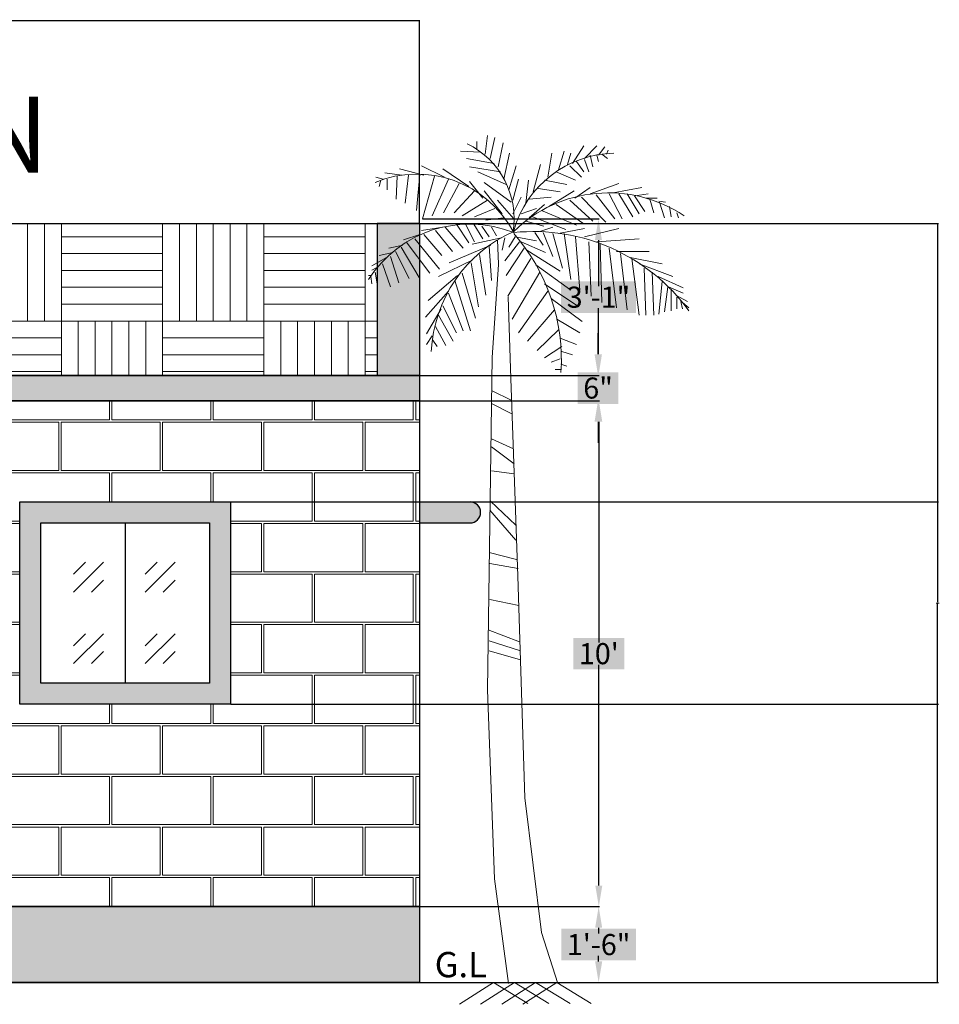
# Model space of a CAD drawing. Units: inches. Extents: x -301 to 715, y -607 to 364.
# Tile 139 of 141: x 497 to 715, y -513 to -279. Entities that reach past the tile are written whole.
import ezdxf

# ---------------------------------------------------------------- set-up
doc = ezdxf.new("R2010")
doc.units = ezdxf.units.IN
doc.header["$MEASUREMENT"] = 0
for name, color, linetype, lineweight in [('A-ANNO-DIMS', 2, 'Continuous', 18), ('A-ANNO-SYMB', 4, 'Continuous', 18), ('A-ANNO-TITL', 1, 'Continuous', 35), ('A-ELEV', 220, 'Continuous', 30), ('A-ELEV-PATT', 4, 'Continuous', 13), ('A-GLAZ', 2, 'Continuous', 25), ('A-GRND', 7, 'Continuous', 25), ('L-PLNT', 94, 'Continuous', 13)]:
    doc.layers.add(name, color=color, linetype=linetype, lineweight=lineweight)
doc.styles.get("Standard").update_dxf_attribs({"font": 'arial.ttf'})
doc.dimstyles.get("Standard").update_dxf_attribs({"dimtxt": 0.18, "dimasz": 0.18, "dimexe": 0.18, "dimexo": 0.0625, "dimgap": 0.09, "dimtad": 0, "dimtih": 1, "dimtoh": 1, "dimdec": 1, "dimzin": 0, "dimdsep": 46, "dimlunit": 4, "dimtxsty": 'Standard', "dimcen": 0.09, "dimclrd": 3, "dimclre": 4, "dimclrt": 6, "dimadec": 0, "dimazin": 0, "dimtfac": 1, "dimtdec": 1, "dimtofl": 0, "dimtmove": 0, "dimatfit": 3, "dimfxl": 1, "dimtfill": 2, "dimtfillclr": 51, "dimtolj": 1, "dimtzin": 0, "dimarcsym": 0})

# ---------------------------------------------------------------- blocks, each defined once
blk = doc.blocks.new('*U34')
for p, q in [((-5.567, 196.707), (-4.987, 201.167)), ((-7.5, 199.68), (-7.5, 197.946)), ((-4.407, 195.716), (-3.247, 200.672)), ((-2.474, 193.733), (-1.315, 199.433)), ((15.116, 194.477), (17.822, 198.689)), ((18.015, 195.716), (20.914, 198.689)), ((-6.727, 197.202), (-11.366, 197.45)), ((-1.121, 190.759), (0.232, 196.955)), ((9.317, 191.255), (10.283, 196.955)), ((11.829, 192.99), (13.182, 197.45)), ((13.956, 194.229), (14.729, 196.955)), ((19.368, 196.459), (19.948, 193.733)), ((20.914, 196.459), (21.301, 194.972)), ((21.301, 196.459), (22.847, 198.441)), ((22.074, 196.707), (23.427, 195.716)), ((23.234, 196.707), (23.62, 197.698)), ((-15.232, 191.255), (-20.644, 193.981)), ((-3.441, 194.477), (-10.013, 195.716)), ((0.038, 188.281), (1.778, 193.981)), ((5.837, 187.786), (7.577, 194.229)), ((14.536, 193.981), (17.242, 191.255)), ((16.082, 194.972), (17.822, 192.494)), ((18.015, 195.468), (18.981, 192.494)), ((-25.283, 191.751), (-29.342, 192.246)), ((-26.443, 191.503), (-26.636, 186.051)), ((-20.064, 191.751), (-25.863, 193.238)), ((-23.737, 191.751), (-24.51, 185.06)), ((-21.031, 191.998), (-21.804, 183.325)), ((-17.551, 191.503), (-20.451, 181.343)), ((-9.433, 189.025), (-15.618, 193.238)), ((-1.894, 192.494), (-9.24, 193.733)), ((-0.541, 189.52), (-7.307, 192.494)), ((11.25, 192.494), (15.889, 190.512)), ((-29.729, 190.759), (-31.469, 191.255)), ((-30.309, 190.512), (-30.695, 189.025)), ((-28.763, 190.759), (-28.763, 188.281)), ((-14.265, 190.759), (-18.131, 182.086)), ((-11.753, 189.768), (-15.425, 182.83)), ((-6.147, 186.299), (-9.24, 190.264)), ((-5.76, 190.016), (0.618, 185.308)), ((1.005, 185.803), (2.358, 190.759)), ((4.098, 185.06), (4.678, 190.512)), ((8.544, 190.512), (13.763, 189.52)), ((19.368, 187.29), (26.133, 189.768)), ((-8.08, 188.034), (-12.912, 182.83)), ((-5.76, 188.034), (-1.508, 182.582)), ((6.997, 188.529), (12.216, 187.786)), ((9.51, 184.317), (15.502, 188.034)), ((15.695, 186.299), (19.368, 188.777)), ((20.721, 187.042), (25.167, 181.343)), ((23.814, 187.29), (26.907, 181.343)), ((24.78, 187.538), (31.546, 188.777)), ((26.133, 187.29), (29.419, 181.838)), ((28.066, 187.29), (30.966, 182.582)), ((29.999, 186.795), (33.092, 187.29)), ((-4.987, 185.803), (-10.979, 182.086)), ((-2.668, 185.803), (1.198, 181.343)), ((1.005, 182.582), (2.938, 186.547)), ((4.871, 186.051), (10.09, 186.547)), ((4.871, 181.591), (8.544, 184.812)), ((11.25, 184.812), (17.628, 180.352)), ((14.536, 185.803), (19.948, 180.847)), ((17.242, 186.547), (23.041, 180.599)), ((29.806, 186.795), (32.319, 183.078)), ((32.512, 186.299), (35.218, 186.299)), ((33.479, 186.051), (34.445, 182.83)), ((35.605, 185.556), (37.151, 185.308)), ((35.798, 185.308), (36.958, 181.591)), ((-3.247, 183.821), (-8.08, 181.838)), ((2.938, 182.582), (6.61, 183.821)), ((7.77, 183.325), (16.082, 179.856)), ((38.118, 184.317), (38.504, 181.838)), ((39.857, 182.83), (40.244, 181.591)), ((-12.332, 180.104), (-9.433, 175.643)), ((-10.206, 180.104), (-8.08, 175.891)), ((-8.273, 180.104), (-6.147, 176.635)), ((-1.315, 181.591), (-5.374, 181.095)), ((-0.348, 180.352), (-1.894, 180.104)), ((4.098, 180.847), (8.35, 179.608)), ((5.644, 181.838), (13.569, 178.865)), ((-21.031, 177.626), (-24.897, 176.387)), ((-15.618, 179.36), (-20.644, 178.617)), ((-20.064, 177.626), (-15.812, 172.67)), ((-17.358, 178.617), (-13.299, 173.661)), ((-15.038, 179.36), (-10.786, 174.404)), ((-6.34, 179.608), (-4.6, 177.13)), ((-4.021, 179.36), (-2.861, 177.378)), ((6.224, 178.121), (8.157, 175.148)), ((7.384, 178.369), (10.476, 179.36)), ((8.157, 178.121), (10.476, 172.422)), ((10.476, 177.874), (12.796, 169.696)), ((11.829, 177.874), (18.015, 179.113)), ((13.182, 177.874), (14.729, 166.97)), ((18.015, 177.13), (26.133, 179.113)), ((-25.09, 175.148), (-28.376, 174.404)), ((-24.317, 175.891), (-18.711, 168.457)), ((-22.191, 176.635), (-16.391, 169.448)), ((-4.214, 175.148), (-14.072, 170.935)), ((-1.701, 176.882), (-8.66, 175.396)), ((-2.668, 176.387), (-2.376, 170.594)), ((-0.928, 176.882), (-1.508, 173.909)), ((2.551, 175.891), (-0.928, 171.431)), ((1.585, 177.13), (0.038, 174.652)), ((1.585, 177.13), (6.61, 176.139)), ((2.938, 175.891), (8.737, 173.413)), ((15.889, 177.13), (16.855, 164.492)), ((18.981, 175.891), (19.561, 163.005)), ((20.914, 175.891), (30.966, 176.635)), ((21.688, 175.396), (22.074, 161.518)), ((-27.409, 173.413), (-30.695, 172.67)), ((-26.829, 173.661), (-23.544, 167.218)), ((-25.476, 174.652), (-21.224, 167.466)), ((-6.92, 172.917), (-5.374, 163.253)), ((-4.6, 174.9), (-4.021, 166.722)), ((3.711, 174.404), (-0.541, 167.961)), ((4.291, 173.909), (12.216, 168.953)), ((23.814, 174.404), (25.554, 160.279)), ((25.554, 173.661), (33.285, 173.661)), ((26.52, 173.165), (28.066, 159.784)), ((-28.956, 172.174), (-32.435, 170.192)), ((-29.922, 170.687), (-27.989, 165.235)), ((-27.989, 172.422), (-26.056, 166.227)), ((-8.466, 171.678), (-16.585, 167.713)), ((-8.853, 170.935), (-7.113, 160.527)), ((5.257, 171.926), (-0.155, 163.005)), ((28.839, 172.174), (36.378, 170.687)), ((29.226, 171.926), (30.966, 158.545)), ((30.966, 170.687), (38.891, 167.713)), ((-31.082, 169.944), (-32.435, 169.2)), ((-31.662, 168.705), (-31.082, 165.483)), ((-10.979, 168.457), (-7.887, 157.801)), ((7.384, 168.705), (0.812, 157.553)), ((6.417, 170.439), (14.729, 164.492)), ((32.126, 169.696), (32.512, 158.545)), ((34.058, 168.705), (34.445, 158.545)), ((-32.628, 167.961), (-33.208, 167.961)), ((-32.628, 167.713), (-32.435, 165.979)), ((-12.139, 167.961), (-19.098, 162.014)), ((-12.719, 166.722), (-9.046, 154.828)), ((8.544, 165.979), (16.662, 160.527)), ((35.412, 167.713), (41.404, 164.988)), ((36.378, 166.474), (35.605, 158.792)), ((-14.265, 164.244), (-19.678, 158.049)), ((-14.265, 163.749), (-10.786, 154.828)), ((9.317, 164.244), (2.358, 154.332)), ((37.731, 165.235), (36.958, 159.288)), ((37.924, 165.235), (41.404, 163.749)), ((38.504, 164.492), (38.504, 159.536)), ((10.09, 162.51), (17.435, 157.058)), ((39.664, 163.253), (42.37, 161.766)), ((39.857, 162.757), (39.857, 160.031)), ((40.824, 161.766), (41.21, 160.031)), ((41.21, 161.518), (42.757, 160.279)), ((-16.005, 160.031), (-19.484, 154.084)), ((-15.618, 160.775), (-12.332, 154.332)), ((10.863, 159.784), (4.484, 152.35)), ((-16.585, 158.545), (-13.106, 152.35)), ((11.443, 157.553), (16.855, 154.332)), ((-17.358, 155.819), (-14.845, 151.358)), ((11.829, 155.075), (6.804, 150.119)), ((-18.131, 153.589), (-19.484, 151.606)), ((-17.938, 152.597), (-16.972, 151.111)), ((12.216, 153.093), (16.082, 151.606)), ((12.603, 151.111), (8.544, 148.385)), ((12.603, 149.872), (15.116, 149.128)), ((12.216, 148.137), (10.09, 147.393)), ((12.409, 145.659), (11.056, 145.659)), ((12.409, 146.898), (13.763, 146.402)), ((-4.081, 140.645), (0.753, 138.261)), ((-4.081, 137.547), (0.753, 135.163)), ((-4.081, 129.205), (1.124, 126.821)), ((-4.081, 127.298), (1.31, 123.246)), ((-4.081, 121.578), (1.31, 120.863)), ((-4.453, 112.283), (1.682, 105.133)), ((-4.267, 114.428), (1.682, 108.708)), ((-4.639, 102.273), (1.868, 100.604)), ((-4.453, 99.651), (2.24, 98.459)), ((-4.453, 91.071), (2.426, 89.641)), ((-4.825, 83.921), (2.612, 81.061)), ((-4.639, 81.299), (2.797, 78.916)), ((-4.639, 78.916), (2.797, 76.771))]:
    blk.add_line(p, q)
for points in [[(-2.363, 170.553), (-3.88, 148.505), (-4.988, 69.634), (-3.325, 24.869), (0, 0)], [(-0.116, 162.848), (0.554, 143.532), (2.217, 96.635), (3.88, 44.054), (7.76, 12.079), (11.64, 0)]]:
    blk.add_lwpolyline(points)
for centre, radius, start, end in [((-18.427, 181.448), 19.715, 350.285, 64.11229), ((25.595, 171.567), 25.395, 91.40319, 163.882), ((-21.738, 166.094), 25.899, 27.67115, 112.5305), ((23.687, 155.341), 32.188, 56.19272, 134.3213), ((-9.259, 151.732), 28.386, 68.38311, 147.5322), ((14.394, 148.393), 32.752, 113.7592, 177.4133), ((5.828, 132.718), 45.639, 35.98777, 95.82273), ((-32.8, 147.923), 45.309, 356.1943, 41.37848)]:
    blk.add_arc(centre, radius, start, end)
blk = doc.blocks.new('*D71')
at = {"layer": 'A-ANNO-DIMS', "color": 0, "lineweight": -2, "transparency": 16777216}
for p, q in [((591.58, -489.55), (634.18, -489.55)), ((634, -494.55), (634, -495.91)), ((634, -502.55), (634, -501.2)), ((591.58, -507.55), (634.18, -507.55))]:
    blk.add_line(p, q, dxfattribs=at)
at = {"layer": 'A-ANNO-DIMS', "color": 0, "transparency": 16777216}
for points in [[(633.17, -494.55), (634.84, -494.55), (634, -489.55)], [(633.17, -502.55), (634.84, -502.55), (634, -507.55)]]:
    blk.add_solid(points, dxfattribs=at)
at = {"layer": 'Defpoints', "color": 0, "transparency": 16777216}
for p in [(591.52, -489.55), (634, -489.55), (591.52, -507.55)]:
    blk.add_point(p, dxfattribs=at)
at = {"layer": 'A-ANNO-DIMS', "color": 0, "transparency": 16777216, "insert": (634, -498.55), "char_height": 5, "attachment_point": 5, "bg_fill": 1, "box_fill_scale": 1.25, "bg_fill_color": 51, "bg_fill_transparency": 0}
blk.add_mtext('\\A1;1\'-6"', dxfattribs=at)
blk = doc.blocks.new('*D72')
at = {"layer": 'A-ANNO-DIMS', "color": 0, "lineweight": -2, "transparency": 16777216}
for p, q in [((591.58, -369.55), (634.22, -369.55)), ((634.04, -374.55), (634.04, -426.91)), ((634.04, -484.55), (634.04, -432.2)), ((591.58, -489.55), (634.22, -489.55))]:
    blk.add_line(p, q, dxfattribs=at)
at = {"layer": 'A-ANNO-DIMS', "color": 0, "transparency": 16777216}
for points in [[(633.21, -374.55), (634.87, -374.55), (634.04, -369.55)], [(633.21, -484.55), (634.87, -484.55), (634.04, -489.55)]]:
    blk.add_solid(points, dxfattribs=at)
at = {"layer": 'Defpoints', "color": 0, "transparency": 16777216}
for p in [(591.52, -369.55), (634.04, -369.55), (591.52, -489.55)]:
    blk.add_point(p, dxfattribs=at)
at = {"layer": 'A-ANNO-DIMS', "color": 0, "transparency": 16777216, "insert": (634.04, -429.55), "char_height": 5, "attachment_point": 5, "bg_fill": 1, "box_fill_scale": 1.25, "bg_fill_color": 51, "bg_fill_transparency": 0}
blk.add_mtext("\\A1;10'", dxfattribs=at)
blk = doc.blocks.new('*D73')
at = {"layer": 'A-ANNO-DIMS', "color": 0, "lineweight": -2, "transparency": 16777216}
for p, q in [((633.86, -358.55), (633.86, -353.55)), ((591.58, -363.55), (634.04, -363.55)), ((591.58, -369.55), (634.04, -369.55)), ((633.86, -374.55), (633.86, -379.55))]:
    blk.add_line(p, q, dxfattribs=at)
at = {"layer": 'A-ANNO-DIMS', "color": 0, "transparency": 16777216}
for points in [[(633.03, -358.55), (634.69, -358.55), (633.86, -363.55)], [(633.03, -374.55), (634.69, -374.55), (633.86, -369.55)]]:
    blk.add_solid(points, dxfattribs=at)
at = {"layer": 'Defpoints', "color": 0, "transparency": 16777216}
for p in [(591.52, -363.55), (633.86, -363.55), (591.52, -369.55)]:
    blk.add_point(p, dxfattribs=at)
at = {"layer": 'A-ANNO-DIMS', "color": 0, "transparency": 16777216, "insert": (633.86, -366.55), "char_height": 5, "attachment_point": 5, "bg_fill": 1, "box_fill_scale": 1.25, "bg_fill_color": 51, "bg_fill_transparency": 0}
blk.add_mtext('\\A1;6"', dxfattribs=at)
blk = doc.blocks.new('*D74')
at = {"layer": 'A-ANNO-DIMS', "color": 0, "lineweight": -2, "transparency": 16777216}
for p, q in [((592.27, -326.45), (634.14, -326.45)), ((633.96, -331.45), (633.96, -342.35)), ((633.96, -358.55), (633.96, -347.64)), ((591.58, -363.55), (634.14, -363.55))]:
    blk.add_line(p, q, dxfattribs=at)
at = {"layer": 'A-ANNO-DIMS', "color": 0, "transparency": 16777216}
for points in [[(633.12, -331.45), (634.79, -331.45), (633.96, -326.45)], [(633.12, -358.55), (634.79, -358.55), (633.96, -363.55)]]:
    blk.add_solid(points, dxfattribs=at)
at = {"layer": 'Defpoints', "color": 0, "transparency": 16777216}
for p in [(592.21, -326.45), (633.96, -326.45), (591.52, -363.55)]:
    blk.add_point(p, dxfattribs=at)
at = {"layer": 'A-ANNO-DIMS', "color": 0, "transparency": 16777216, "insert": (633.96, -345), "char_height": 5, "attachment_point": 5, "bg_fill": 1, "box_fill_scale": 1.25, "bg_fill_color": 51, "bg_fill_transparency": 0}
blk.add_mtext('\\A1;3\'-1"', dxfattribs=at)
blk = doc.blocks.new('GRADE-MARK-4')
for p, q in [((8.05, 5.16), (0, 0)), ((13.05, 5.16), (5, 0)), ((8.05, 5.16), (16.2, 0.15)), ((18.05, 5.16), (10, 0)), ((13.05, 5.16), (21.2, 0.15)), ((23.05, 5.16), (15, 0)), ((18.05, 5.16), (26.2, 0.15)), ((23.05, 5.16), (31.2, 0.15))]:
    blk.add_line(p, q)
blk = doc.blocks.new('*D192')
at = {"layer": 'A-ANNO-DIMS', "color": 4, "lineweight": -2, "transparency": 16777216}
for p, q in [((254.02, -327.49), (254.02, -279.27)), ((591.52, -327.49), (591.52, -279.27))]:
    blk.add_line(p, q, dxfattribs=at)
at = {"layer": 'A-ANNO-DIMS', "color": 3, "lineweight": -2, "transparency": 16777216}
for p, q in [((254.2, -279.45), (422.16, -279.45)), ((591.34, -279.45), (423.38, -279.45))]:
    blk.add_line(p, q, dxfattribs=at)
at = {"layer": 'A-ANNO-DIMS', "color": 3, "transparency": 16777216}
for points in [[(254.2, -279.42), (254.2, -279.48), (254.02, -279.45)], [(591.34, -279.42), (591.34, -279.48), (591.52, -279.45)]]:
    blk.add_solid(points, dxfattribs=at)
at = {"layer": 'Defpoints', "color": 0, "transparency": 16777216}
for p in [(591.52, -279.45), (254.02, -327.55), (591.52, -327.55)]:
    blk.add_point(p, dxfattribs=at)
at = {"layer": 'A-ANNO-DIMS', "color": 6, "transparency": 16777216, "insert": (422.77, -279.45), "char_height": 0.18, "attachment_point": 5, "bg_fill": 1, "box_fill_scale": 1.25, "bg_fill_color": 51, "bg_fill_transparency": 0}
blk.add_mtext('\\A1;28\'-1 1/2"', dxfattribs=at)
blk = doc.blocks.new('*D193')
at = {"layer": 'A-ANNO-DIMS', "color": 4, "lineweight": -2, "transparency": 16777216}
for p, q in [((591.58, -327.55), (714.54, -327.55)), ((591.58, -507.55), (714.54, -507.55))]:
    blk.add_line(p, q, dxfattribs=at)
at = {"layer": 'A-ANNO-DIMS', "color": 3, "lineweight": -2, "transparency": 16777216}
for p, q in [((714.36, -327.73), (714.36, -417.37)), ((714.36, -507.37), (714.36, -417.73))]:
    blk.add_line(p, q, dxfattribs=at)
at = {"layer": 'A-ANNO-DIMS', "color": 3, "transparency": 16777216}
for points in [[(714.33, -327.73), (714.39, -327.73), (714.36, -327.55)], [(714.33, -507.37), (714.39, -507.37), (714.36, -507.55)]]:
    blk.add_solid(points, dxfattribs=at)
at = {"layer": 'Defpoints', "color": 0, "transparency": 16777216}
for p in [(591.52, -327.55), (714.36, -327.55), (591.52, -507.55)]:
    blk.add_point(p, dxfattribs=at)
at = {"layer": 'A-ANNO-DIMS', "color": 6, "transparency": 16777216, "insert": (714.36, -417.55), "char_height": 0.18, "attachment_point": 5, "bg_fill": 1, "box_fill_scale": 1.25, "bg_fill_color": 51, "bg_fill_transparency": 0}
blk.add_mtext('\\A1;15\'-0"', dxfattribs=at)
blk = doc.blocks.new('*D199')
at = {"layer": 'A-ANNO-DIMS', "color": 4, "lineweight": -2, "transparency": 16777216}
for p, q in [((546.83, -393.55), (714.54, -393.55)), ((546.83, -441.55), (714.54, -441.55))]:
    blk.add_line(p, q, dxfattribs=at)
at = {"layer": 'A-ANNO-DIMS', "color": 3, "lineweight": -2, "transparency": 16777216}
for p, q in [((714.36, -393.73), (714.36, -417.37)), ((714.36, -441.37), (714.36, -417.73))]:
    blk.add_line(p, q, dxfattribs=at)
at = {"layer": 'A-ANNO-DIMS', "color": 3, "transparency": 16777216}
for points in [[(714.33, -393.73), (714.39, -393.73), (714.36, -393.55)], [(714.33, -441.37), (714.39, -441.37), (714.36, -441.55)]]:
    blk.add_solid(points, dxfattribs=at)
at = {"layer": 'Defpoints', "color": 0, "transparency": 16777216}
for p in [(546.77, -393.55), (546.77, -441.55), (714.36, -441.55)]:
    blk.add_point(p, dxfattribs=at)
at = {"layer": 'A-ANNO-DIMS', "color": 6, "transparency": 16777216, "insert": (714.36, -417.55), "char_height": 0.18, "attachment_point": 5, "bg_fill": 1, "box_fill_scale": 1.25, "bg_fill_color": 51, "bg_fill_transparency": 0}
blk.add_mtext('\\A1;4\'-0"', dxfattribs=at)

msp = doc.modelspace()

# ---------------------------------------------------------------- hatches: boundary and pattern name
at = {"layer": 'A-ELEV-PATT'}
h = msp.add_hatch(dxfattribs=at)
h.set_pattern_fill('AR-RROOF', color=256, scale=2)
h.set_pattern_definition([(0, (458.6211, 9.3248), (4.4, 2), [30, -4, 10, -2]), (0, (461.281, 10.3248), (-2, 2.66), [6, -0.66, 12, -1.5]), (0, (459.6211, 11.0248), (10.4, 1.34), [16, -2.8, 8, -2])])
h.paths.add_polyline_path([(254.02, -363.55), (264.02, -363.55), (264.02, -327.55), (254.02, -327.55)])
h.paths.add_polyline_path([(591.52, -327.55), (581.52, -327.55), (581.52, -363.55), (591.52, -363.55)])
h = msp.add_hatch(dxfattribs=at)
h.set_pattern_fill('AR-PARQ1', color=256, scale=2)
h.set_pattern_definition([(90, (458.62, 9.325), (-24, 24), [24, -24]), (90, (462.62, 9.325), (-24, 24), [24, -24]), (90, (466.62, 9.325), (-24, 24), [24, -24]), (90, (470.62, 9.325), (-24, 24), [24, -24]), (90, (474.62, 9.325), (-24, 24), [24, -24]), (90, (478.62, 9.325), (-24, 24), [24, -24]), (90, (482.62, 9.325), (-24, 24), [24, -24]), (0, (458.62, 33.325), (24, -24), [24, -24]), (0, (458.62, 37.325), (24, -24), [24, -24]), (0, (458.62, 41.325), (24, -24), [24, -24]), (0, (458.62, 45.325), (24, -24), [24, -24]), (0, (458.62, 49.325), (24, -24), [24, -24]), (0, (458.62, 53.325), (24, -24), [24, -24]), (0, (458.62, 57.325), (24, -24), [24, -24])])
h.paths.add_polyline_path([(264.02, -327.55), (264.02, -363.55), (581.52, -363.55), (581.52, -327.55)])
h = msp.add_hatch(color=256, dxfattribs=at)
h.dxf.hatch_style = 1
h.paths.add_polyline_path([(591.52, -363.55), (254.02, -363.55), (254.02, -369.55), (591.52, -369.55)])
h.paths.add_polyline_path([(461.02, -393.55), (413.02, -393.55), (413.02, -489.55), (461.02, -489.55)])
h.paths.add_polyline_path([(456.02, -398.55), (456.02, -484.55), (418.02, -484.55), (418.02, -398.55)], flags=16)
h.paths.add_polyline_path([(546.77, -393.55), (496.77, -393.55), (496.77, -441.55), (546.77, -441.55)])
h.paths.add_polyline_path([(501.77, -398.55), (541.77, -398.55), (541.77, -436.55), (501.77, -436.55)], flags=16)
h.paths.add_polyline_path([(360.02, -393.55), (310.02, -393.55), (310.02, -441.55), (360.02, -441.55)])
h.paths.add_polyline_path([(355.02, -398.55), (355.02, -436.55), (315.02, -436.55), (315.02, -398.55)], flags=16)
h = msp.add_hatch(dxfattribs=at)
h.set_pattern_fill('AR-B816C', color=256, scale=1.5)
h.set_pattern_definition([(0, (458.621, 9.325), (12, 12), [23.4375, -0.5625]), (0, (446.621, 9.887), (12, 12), [23.4375, -0.5625]), (90, (458.621, 9.325), (-12, 12), [-12.5625, 11.4375]), (90, (458.059, 9.325), (-12, 12), [-12.5625, 11.4375])])
h.paths.add_polyline_path([(254.02, -489.55), (413.02, -489.55), (413.02, -393.55), (461.02, -393.55), (461.02, -489.55), (591.52, -489.55), (591.52, -369.55), (254.02, -369.55)])
h.paths.add_polyline_path([(310.02, -393.55), (360.02, -393.55), (360.02, -441.55), (310.02, -441.55)], flags=16)
h.paths.add_polyline_path([(315.02, -398.55), (355.02, -398.55), (355.02, -436.55), (315.02, -436.55)], flags=0)
h.paths.add_polyline_path([(496.77, -393.55), (546.77, -393.55), (546.77, -441.55), (496.77, -441.55)], flags=16)
h.paths.add_polyline_path([(501.77, -398.55), (541.77, -398.55), (541.77, -436.55), (501.77, -436.55)], flags=0)
h = msp.add_hatch(color=256, dxfattribs=at)
h.dxf.hatch_style = 1
h.paths.add_polyline_path([(242.02, -393.55, 1), (242.02, -398.55), (254.02, -398.55), (254.02, -393.55)])
h.paths.add_polyline_path([(603.52, -398.55, 1), (603.52, -393.55), (591.52, -393.55), (591.52, -398.55)])
h = msp.add_hatch(dxfattribs=at)
h.set_pattern_fill('GOST_GLASS', color=256, scale=2)
h.set_pattern_definition([(45, (458.621, 9.325), (16.97056, -2e-15), [10, -14]), (45, (462.864, 9.325), (16.97056, -2e-15), [4, -20]), (45, (458.621, 13.567), (16.97056, -2e-15), [4, -20])])
h.paths.add_polyline_path([(335.02, -398.55), (315.02, -398.55), (315.02, -436.55), (335.02, -436.55)])
h.paths.add_polyline_path([(355.02, -398.55), (335.02, -398.55), (335.02, -436.55), (355.02, -436.55)])
h.paths.add_polyline_path([(521.77, -398.55), (501.77, -398.55), (501.77, -436.55), (521.77, -436.55)])
h.paths.add_polyline_path([(541.77, -398.55), (521.77, -398.55), (521.77, -436.55), (541.77, -436.55)])
h = msp.add_hatch(dxfattribs=at)
h.set_pattern_fill('AR-CONC', color=256, scale=2)
h.set_pattern_definition([(50, (458.621, 9.325), (14.3452, -1.25504), [1.5, -16.5]), (355, (458.621, 9.325), (-2.77503, 15.04384), [1.2, -13.2]), (100.4514, (459.817, 9.22), (11.57018, 13.7888), [1.2748, -14.02284]), (46.1842, (458.621, 13.325), (21.3448, -3.3104), [2.25, -24.75]), (96.6356, (460.4, 13.049), (18.69324, 19.4824), [1.9122, -21.0343]), (351.184, (458.62, 13.325), (18.6932, 19.4824), [1.8, -19.8]), (21, (460.621, 12.325), (11.93814, -8.05238), [1.5, -16.5]), (326, (460.621, 12.325), (4.8663, 14.503), [1.2, -13.2]), (71.4514, (461.616, 11.654), (16.80445, 6.45062), [1.2748, -14.02284]), (37.5, (458.621, 9.325), (0.243197, 6.657877), [0, -13.04, 0, -13.4, 0, -13.25]), (7.5, (458.621, 9.325), (5.26139, 7.88823), [0, -7.64, 0, -12.74, 0, -5.05]), (327.5, (454.161, 9.325), (10.67645, -0.4511), [0, -5, 0, -15.6, 0, -20.7]), (317.5, (452.161, 9.325), (11.66372, 2.0021), [0, -6.5, 0, -10.36, 0, -14.7])])
h.paths.add_polyline_path([(254.02, -489.55), (254.02, -507.55), (413.02, -507.55), (413.02, -489.55)])
h.paths.add_polyline_path([(591.52, -507.55), (591.52, -489.55), (461.02, -489.55), (461.02, -507.55)])

# ---------------------------------------------------------------- linework, layer by layer
at = {"layer": 'A-ELEV'}
for p, q in [((254.02, -327.55), (591.52, -327.55)), ((591.52, -327.55), (581.52, -327.55)), ((581.52, -327.55), (581.52, -363.55)), ((254.02, -363.55), (591.52, -363.55)), ((254.02, -369.55), (591.52, -369.55)), ((591.48, -393.55), (603.52, -393.55)), ((591.48, -398.55), (603.52, -398.55)), ((254.02, -489.55), (591.52, -489.55)), ((254.02, -507.55), (591.52, -507.55))]:
    msp.add_line(p, q, dxfattribs=at)
for points in [[(254.02, -327.55), (591.52, -327.55), (591.52, -363.55), (254.02, -363.55)], [(254.02, -363.55), (591.52, -363.55), (591.52, -369.55), (254.02, -369.55)], [(254.02, -369.55), (591.52, -369.55), (591.52, -489.55), (254.02, -489.55)], [(254.02, -489.55), (591.52, -489.55), (591.52, -507.55), (254.02, -507.55)]]:
    msp.add_lwpolyline(points, close=True, dxfattribs=at)
msp.add_arc((603.52, -396.05), 2.5, 270, 90, dxfattribs=at)
at = {"layer": 'A-GLAZ'}
msp.add_line((521.77, -398.55), (521.77, -436.55), dxfattribs=at)
for points in [[(496.77, -393.55), (546.77, -393.55), (546.77, -441.55), (496.77, -441.55)], [(501.77, -398.55), (541.77, -398.55), (541.77, -436.55), (501.77, -436.55)]]:
    msp.add_lwpolyline(points, close=True, dxfattribs=at)
at = {"layer": 'A-GRND'}
msp.add_line((591.52, -507.55), (639.52, -507.55), dxfattribs=at)

# ---------------------------------------------------------------- block references
at = {"layer": 'A-ANNO-SYMB'}
msp.add_blockref('GRADE-MARK-4', (601.02, -512.71), dxfattribs=at)
at = {"layer": 'L-PLNT'}
msp.add_blockref('*U34', (612.66, -507.79), dxfattribs=at)

# ---------------------------------------------------------------- texts
at = {"layer": 'A-ANNO-SYMB'}
msp.add_text('G.L', height=6, dxfattribs=at).set_placement((595.14, -506.3))
at = {"layer": 'A-ANNO-TITL'}
msp.add_text('ELEVATION', height=18, dxfattribs=at).set_placement((374.43, -315.47))

# ---------------------------------------------------------------- dimensions: what is measured, and where the dimension line sits
at = {"layer": 'A-ANNO-DIMS'}
dim = msp.add_linear_dim(base=(591.52, -279.45), p1=(254.02, -327.55), p2=(591.52, -327.55), dimstyle='Standard', override={"dimdec": 1, "dimlfac": 1, "dimrnd": 0, "dimzin": 1, "dimdsep": 46, "dimlunit": 4, "dimfrac": 2}, dxfattribs=at)
dim.commit()
dim.dimension.update_dxf_attribs({"geometry": '*D192', "text_midpoint": (422.77, -279.45)})
for base, p1, p2, override, picture, middle in [((633.96, -326.45), (591.52, -363.55), (592.21, -326.45), {"dimtxt": 5, "dimasz": 5, "dimclrd": 0, "dimclre": 0, "dimclrt": 0}, '*D74', (633.96, -345)), ((714.36, -327.55), (591.52, -507.55), (591.52, -327.55), {"dimdec": 1, "dimlfac": 1, "dimrnd": 0, "dimzin": 1, "dimdsep": 46, "dimlunit": 4, "dimfrac": 2}, '*D193', (714.36, -417.55)), ((633.86, -363.55), (591.52, -369.55), (591.52, -363.55), {"dimtxt": 5, "dimasz": 5, "dimclrd": 0, "dimclre": 0, "dimclrt": 0}, '*D73', (633.86, -366.55)), ((634.04, -369.55), (591.52, -489.55), (591.52, -369.55), {"dimtxt": 5, "dimasz": 5, "dimclrd": 0, "dimclre": 0, "dimclrt": 0}, '*D72', (634.04, -429.55)), ((714.36, -441.55), (546.77, -393.55), (546.77, -441.55), {"dimdec": 1, "dimlfac": 1, "dimrnd": 0, "dimzin": 1, "dimdsep": 46, "dimlunit": 4, "dimfrac": 2}, '*D199', (714.36, -417.55)), ((634, -489.55), (591.52, -507.55), (591.52, -489.55), {"dimtxt": 5, "dimasz": 5, "dimclrd": 0, "dimclre": 0, "dimclrt": 0}, '*D71', (634, -498.55))]:
    dim = msp.add_linear_dim(base=base, p1=p1, p2=p2, angle=90, dimstyle='Standard', override=override, dxfattribs=at)
    dim.commit()
    dim.dimension.update_dxf_attribs({"geometry": picture, "text_midpoint": middle})

doc.saveas('drawing.dxf')
